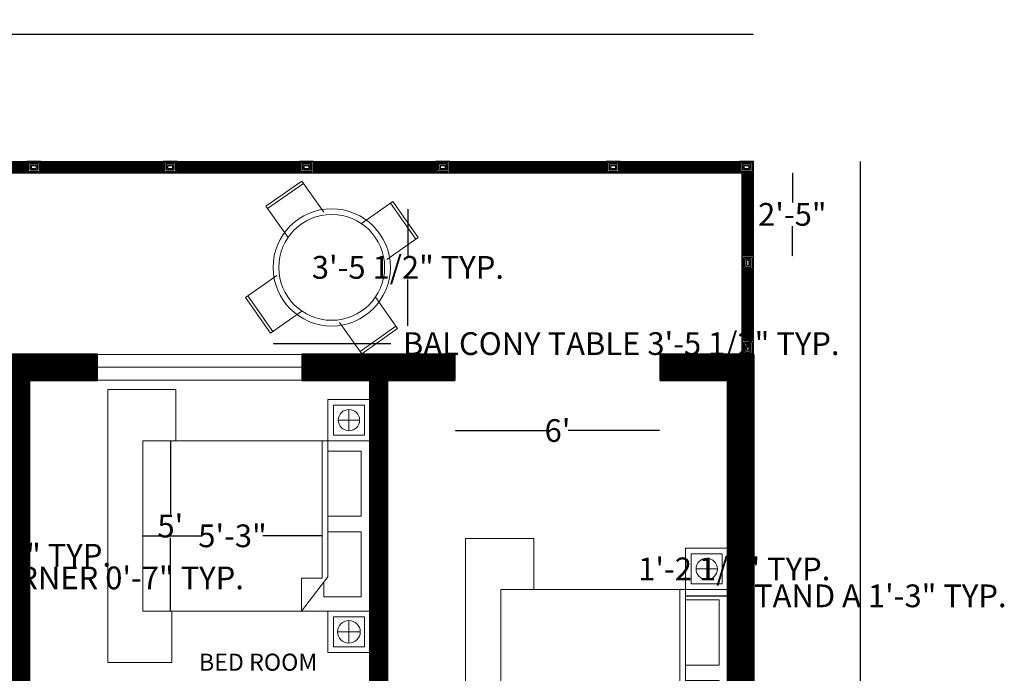
# Model space of a CAD drawing. Units: inches. Extents: x 348 to 1197, y 2602 to 3078.
# Tile 4 of 4: x 850 to 1197, y 2848 to 3078. Entities that reach past the tile are written whole.
import ezdxf

# ---------------------------------------------------------------- set-up
doc = ezdxf.new("R2010")
doc.units = ezdxf.units.IN
doc.header["$MEASUREMENT"] = 0
for name, color, linetype, lineweight in [('A-ANNO-DIMS', 20, 'Continuous', 18), ('A-AREA-IDEN', 104, 'Continuous', 18), ('A-WALL-PATT', 250, 'Continuous', 13), ('balcony', 201, 'Continuous', 25), ('bed', 5, 'Continuous', 18), ('table', 6, 'Continuous', 18), ('walls', 4, 'Continuous', 50), ('windows', 2, 'Continuous', 18)]:
    doc.layers.add(name, color=color, linetype=linetype, lineweight=lineweight)
doc.styles.get("Standard").update_dxf_attribs({"font": 'arial.ttf'})
doc.dimstyles.get("Standard").update_dxf_attribs({"dimtxt": 8, "dimasz": 0.18, "dimexe": 0.18, "dimexo": 0.0625, "dimgap": 0.09, "dimtad": 0, "dimtih": 1, "dimtoh": 1, "dimdec": 0, "dimzin": 0, "dimdsep": 46, "dimlunit": 3, "dimtxsty": 'Standard', "dimblk": 'DOT', "dimcen": 0.09, "dimse1": 1, "dimse2": 1, "dimadec": 0, "dimazin": 0, "dimtfac": 1, "dimtdec": 0, "dimtofl": 0, "dimtmove": 0, "dimatfit": 3, "dimfxl": 1, "dimtolj": 1, "dimtzin": 0, "dimarcsym": 0})

# ---------------------------------------------------------------- blocks, each defined once
blk = doc.blocks.new('*U16')
at = {"layer": 'table'}
for p, q in [((-7.7, -6.73), (-7.7, 6.73)), ((-7.7, 6.73), (7.7, 6.73)), ((-7.7, 5.73), (7.7, 5.73)), ((7.7, 6.73), (7.7, -6.73))]:
    blk.add_line(p, q, dxfattribs=at)
blk = doc.blocks.new('*U17')
at = {"layer": 'table', "transparency": 16777216}
blk.add_blockref('*U16', (596.31, 3015.18), dxfattribs=at)
for p, rotation in [((570.95, 2992.17), 90), ((619.32, 2989.82), 270), ((593.96, 2966.81), 180)]:
    blk.add_blockref('*U16', p, dxfattribs=dict(at, rotation=rotation))
blk = doc.blocks.new('_Dot')
at = {"color": 0, "linetype": 'ByBlock', "lineweight": -2}
blk.add_line((-0.5, 0), (-1, 0), dxfattribs=at)
at = {"color": 0, "linetype": 'ByBlock', "const_width": 0.5}
blk.add_lwpolyline([(-0.25, 0, 1), (0.25, 0, 1)], format="xyb", close=True, dxfattribs=at)
blk = doc.blocks.new('*D21')
at = {"layer": 'A-ANNO-DIMS', "color": 0, "lineweight": -2, "transparency": 16777216}
for p, q in [((1122, 3023.99), (1122, 3013.7)), ((1122, 2995.07), (1122, 3005.35))]:
    blk.add_line(p, q, dxfattribs=at)
at = {"layer": 'Defpoints', "color": 0, "transparency": 16777216}
for p in [(1108.32, 3024.17), (1122, 3024.17), (1108.32, 2994.89)]:
    blk.add_point(p, dxfattribs=at)
at = {"layer": 'A-ANNO-DIMS', "color": 0, "lineweight": -2, "transparency": 16777216, "xscale": 0.18, "yscale": 0.18, "zscale": 0.18}
for p, rotation in [((1122, 3024.17), 90), ((1122, 2994.89), 270)]:
    blk.add_blockref('_Dot', p, dxfattribs=dict(at, rotation=rotation))
at = {"layer": 'A-ANNO-DIMS', "color": 0, "transparency": 16777216, "insert": (1122, 3009.53), "char_height": 8, "attachment_point": 5}
blk.add_mtext('\\A1;2\'-5"', dxfattribs=at)
blk = doc.blocks.new('*D22')
at = {"layer": 'A-ANNO-DIMS', "color": 0, "lineweight": -2, "transparency": 16777216}
for p, q in [((1003.5, 2933.44), (1035.52, 2933.44)), ((1075.14, 2933.44), (1043.11, 2933.44))]:
    blk.add_line(p, q, dxfattribs=at)
at = {"layer": 'Defpoints', "color": 0, "transparency": 16777216}
for p in [(1003.32, 2955.7), (1075.32, 2955.7), (1003.32, 2933.44)]:
    blk.add_point(p, dxfattribs=at)
at = {"layer": 'A-ANNO-DIMS', "color": 0, "lineweight": -2, "transparency": 16777216, "xscale": 0.18, "yscale": 0.18, "zscale": 0.18, "rotation": 180}
blk.add_blockref('_Dot', (1003.32, 2933.44), dxfattribs=at)
at = {"layer": 'A-ANNO-DIMS', "color": 0, "lineweight": -2, "transparency": 16777216, "xscale": 0.18, "yscale": 0.18, "zscale": 0.18}
blk.add_blockref('_Dot', (1075.32, 2933.44), dxfattribs=at)
at = {"layer": 'A-ANNO-DIMS', "color": 0, "transparency": 16777216, "insert": (1039.32, 2933.44), "char_height": 8, "attachment_point": 5}
blk.add_mtext("\\A1;6'", dxfattribs=at)
blk = doc.blocks.new('*D33')
at = {"layer": 'A-ANNO-DIMS', "color": 0, "lineweight": -2, "transparency": 16777216}
for p, q in [((893.5, 2896.39), (914.14, 2896.39)), ((956.24, 2896.39), (935.59, 2896.39))]:
    blk.add_line(p, q, dxfattribs=at)
at = {"layer": 'Defpoints', "color": 0, "transparency": 16777216}
for p in [(893.32, 2899.84), (956.42, 2896.39), (956.42, 2896.39)]:
    blk.add_point(p, dxfattribs=at)
at = {"layer": 'A-ANNO-DIMS', "color": 0, "lineweight": -2, "transparency": 16777216, "xscale": 0.18, "yscale": 0.18, "zscale": 0.18, "rotation": 180}
blk.add_blockref('_Dot', (893.32, 2896.39), dxfattribs=at)
at = {"layer": 'A-ANNO-DIMS', "color": 0, "lineweight": -2, "transparency": 16777216, "xscale": 0.18, "yscale": 0.18, "zscale": 0.18}
blk.add_blockref('_Dot', (956.42, 2896.39), dxfattribs=at)
at = {"layer": 'A-ANNO-DIMS', "color": 0, "transparency": 16777216, "insert": (924.87, 2896.39), "char_height": 8, "attachment_point": 5}
blk.add_mtext('\\A1;5\'-3"', dxfattribs=at)
blk = doc.blocks.new('*D34')
at = {"layer": 'A-ANNO-DIMS', "color": 0, "lineweight": -2, "transparency": 16777216}
for p, q in [((902.98, 2929.66), (902.98, 2903.99)), ((902.98, 2870.02), (902.98, 2895.68))]:
    blk.add_line(p, q, dxfattribs=at)
at = {"layer": 'Defpoints', "color": 0, "transparency": 16777216}
for p in [(902.98, 2929.84), (933.32, 2929.84), (937.33, 2869.84)]:
    blk.add_point(p, dxfattribs=at)
at = {"layer": 'A-ANNO-DIMS', "color": 0, "lineweight": -2, "transparency": 16777216, "xscale": 0.18, "yscale": 0.18, "zscale": 0.18}
for p, rotation in [((902.98, 2929.84), 90), ((902.98, 2869.84), 270)]:
    blk.add_blockref('_Dot', p, dxfattribs=dict(at, rotation=rotation))
at = {"layer": 'A-ANNO-DIMS', "color": 0, "transparency": 16777216, "insert": (902.98, 2899.84), "char_height": 8, "attachment_point": 5}
blk.add_mtext("\\A1;5'", dxfattribs=at)
blk = doc.blocks.new('BED-QUEEN')
for p, q in [((24, 96), (0, 96)), ((0, 96), (0, 0)), ((24, 78), (24, 96)), ((92.39, 78), (12.39, 78)), ((12.39, 78), (12.39, 18)), ((75.49, 78), (75.49, 29.69)), ((77.49, 78), (77.49, 30.16)), ((77.49, 30.16), (68.23, 18)), ((68.23, 29.62), (75.49, 29.69)), ((68.23, 18), (68.23, 29.62)), ((12.39, 18), (92.39, 18)), ((22.56, 18), (22.56, 0)), ((22.56, 0), (0, 0))]:
    blk.add_line(p, q)
for points in [[(77.49, 51.42), (89.26, 51.42), (89.26, 74.34), (77.49, 74.34)], [(76.09, 28.32), (76.09, 23.06), (89.26, 23.06), (89.26, 45.98), (77.49, 45.98)]]:
    blk.add_lwpolyline(points)
blk = doc.blocks.new('NIGHTSTAND-LAMP-A')
for p, q in [((7.45, 11), (7.45, 3.51)), ((3.7, 7.26), (11.2, 7.26))]:
    blk.add_line(p, q)
for points in [[(14.9, 0), (0, 0), (0, 14.51), (14.9, 14.51)], [(12.9, 2), (2, 2), (2, 12.51), (12.9, 12.51)]]:
    blk.add_lwpolyline(points, close=True)
blk.add_circle((7.45, 7.26), 3.75)
blk = doc.blocks.new('NIGHTSTAND-LAMP-B')
for p, q in [((7.45, 11.24), (7.45, 3.27)), ((11.44, 7.26), (3.46, 7.26))]:
    blk.add_line(p, q)
for points in [[(14.9, 0), (0, 0), (0, 14.51), (14.9, 14.51)], [(12.9, 2), (2, 2), (2, 12.51), (12.9, 12.51)]]:
    blk.add_lwpolyline(points, close=True)
blk.add_circle((7.45, 7.26), 3.99)
blk = doc.blocks.new('RAIL-POST-CORE')
for points in [[(0, 0), (3, 0), (3, 3.9), (0, 3.9)], [(0.5, 0.5), (2.5, 0.5), (2.5, 3.4), (0.5, 3.4)], [(1, 1), (2, 1), (2, 2.9), (1, 2.9)]]:
    blk.add_lwpolyline(points, close=True)
blk = doc.blocks.new('BALCONY-TABLE-ROUND')
for radius in [20.64, 18.64]:
    blk.add_circle((20.64, 20.64), radius)
blk = doc.blocks.new('*D52')
at = {"layer": 'A-ANNO-DIMS', "color": 0, "lineweight": -2, "transparency": 16777216}
for p, q in [((939.34, 2964.05), (980.26, 2964.05)), ((980.44, 2964.05), (980.62, 2964.05))]:
    blk.add_line(p, q, dxfattribs=at)
at = {"layer": 'Defpoints', "color": 0, "transparency": 16777216}
for p in [(939.16, 2970.24), (980.44, 2970.24), (980.44, 2964.05)]:
    blk.add_point(p, dxfattribs=at)
at = {"layer": 'A-ANNO-DIMS', "color": 0, "lineweight": -2, "transparency": 16777216, "xscale": 0.18, "yscale": 0.18, "zscale": 0.18, "rotation": 180}
blk.add_blockref('_Dot', (939.16, 2964.05), dxfattribs=at)
at = {"layer": 'A-ANNO-DIMS', "color": 0, "lineweight": -2, "transparency": 16777216, "xscale": 0.18, "yscale": 0.18, "zscale": 0.18}
blk.add_blockref('_Dot', (980.44, 2964.05), dxfattribs=at)
at = {"layer": 'A-ANNO-DIMS', "color": 0, "transparency": 16777216, "insert": (1061.75, 2964.05), "char_height": 8, "attachment_point": 5}
blk.add_mtext('\\A1;BALCONY TABLE 3\'-5 1/2" TYP.', dxfattribs=at)
blk = doc.blocks.new('*D53')
at = {"layer": 'A-ANNO-DIMS', "color": 0, "lineweight": -2, "transparency": 16777216}
for p, q in [((986.63, 3011.33), (986.63, 2995.1)), ((986.63, 2970.42), (986.63, 2986.65))]:
    blk.add_line(p, q, dxfattribs=at)
at = {"layer": 'Defpoints', "color": 0, "transparency": 16777216}
for p in [(980.44, 3011.51), (986.63, 3011.51), (980.44, 2970.24)]:
    blk.add_point(p, dxfattribs=at)
at = {"layer": 'A-ANNO-DIMS', "color": 0, "lineweight": -2, "transparency": 16777216, "xscale": 0.18, "yscale": 0.18, "zscale": 0.18}
for p, rotation in [((986.63, 3011.51), 90), ((986.63, 2970.24), 270)]:
    blk.add_blockref('_Dot', p, dxfattribs=dict(at, rotation=rotation))
at = {"layer": 'A-ANNO-DIMS', "color": 0, "transparency": 16777216, "insert": (986.63, 2990.88), "char_height": 8, "attachment_point": 5}
blk.add_mtext('\\A1;3\'-5 1/2" TYP.', dxfattribs=at)
blk = doc.blocks.new('*D62')
at = {"layer": 'A-ANNO-DIMS', "color": 0, "lineweight": -2, "transparency": 16777216}
for p, q in [((825.4, 2881.58), (831.83, 2881.58)), ((832.01, 2881.58), (832.19, 2881.58))]:
    blk.add_line(p, q, dxfattribs=at)
at = {"layer": 'Defpoints', "color": 0, "transparency": 16777216}
for p in [(825.22, 2882.6), (832.01, 2882.6), (832.01, 2881.58)]:
    blk.add_point(p, dxfattribs=at)
at = {"layer": 'A-ANNO-DIMS', "color": 0, "lineweight": -2, "transparency": 16777216, "xscale": 0.18, "yscale": 0.18, "zscale": 0.18, "rotation": 180}
blk.add_blockref('_Dot', (825.22, 2881.58), dxfattribs=at)
at = {"layer": 'A-ANNO-DIMS', "color": 0, "lineweight": -2, "transparency": 16777216, "xscale": 0.18, "yscale": 0.18, "zscale": 0.18}
blk.add_blockref('_Dot', (832.01, 2881.58), dxfattribs=at)
at = {"layer": 'A-ANNO-DIMS', "color": 0, "transparency": 16777216, "insert": (881.63, 2881.58), "char_height": 8, "attachment_point": 5}
blk.add_mtext('\\A1;BURNER 0\'-7" TYP.', dxfattribs=at)
blk = doc.blocks.new('*D63')
at = {"layer": 'A-ANNO-DIMS', "color": 0, "lineweight": -2, "transparency": 16777216}
for p, q in [((833.03, 2889.38), (833.03, 2889.56)), ((833.03, 2889.56), (833.21, 2889.56)), ((833.03, 2882.78), (833.03, 2889.2))]:
    blk.add_line(p, q, dxfattribs=at)
at = {"layer": 'Defpoints', "color": 0, "transparency": 16777216}
for p in [(832.01, 2889.38), (833.03, 2889.38), (832.01, 2882.6)]:
    blk.add_point(p, dxfattribs=at)
at = {"layer": 'A-ANNO-DIMS', "color": 0, "lineweight": -2, "transparency": 16777216, "xscale": 0.18, "yscale": 0.18, "zscale": 0.18}
for p, rotation in [((833.03, 2889.38), 90), ((833.03, 2882.6), 270)]:
    blk.add_blockref('_Dot', p, dxfattribs=dict(at, rotation=rotation))
at = {"layer": 'A-ANNO-DIMS', "color": 0, "transparency": 16777216, "insert": (857.68, 2889.56), "char_height": 8, "attachment_point": 5}
blk.add_mtext('\\A1;0\'-7" TYP.', dxfattribs=at)
blk = doc.blocks.new('*D64')
at = {"layer": 'A-ANNO-DIMS', "color": 0, "lineweight": -2, "transparency": 16777216}
for p, q in [((1084.6, 2875.26), (1099.14, 2875.26)), ((1099.32, 2875.26), (1099.5, 2875.26))]:
    blk.add_line(p, q, dxfattribs=at)
at = {"layer": 'Defpoints', "color": 0, "transparency": 16777216}
for p in [(1084.42, 2877.5), (1099.32, 2877.5), (1099.32, 2875.26)]:
    blk.add_point(p, dxfattribs=at)
at = {"layer": 'A-ANNO-DIMS', "color": 0, "lineweight": -2, "transparency": 16777216, "xscale": 0.18, "yscale": 0.18, "zscale": 0.18, "rotation": 180}
blk.add_blockref('_Dot', (1084.42, 2875.26), dxfattribs=at)
at = {"layer": 'A-ANNO-DIMS', "color": 0, "lineweight": -2, "transparency": 16777216, "xscale": 0.18, "yscale": 0.18, "zscale": 0.18}
blk.add_blockref('_Dot', (1099.32, 2875.26), dxfattribs=at)
at = {"layer": 'A-ANNO-DIMS', "color": 0, "transparency": 16777216, "insert": (1149.72, 2875.26), "char_height": 8, "attachment_point": 5}
blk.add_mtext('\\A1;STAND A 1\'-3" TYP.', dxfattribs=at)
blk = doc.blocks.new('*D65')
at = {"layer": 'A-ANNO-DIMS', "color": 0, "lineweight": -2, "transparency": 16777216}
for p, q in [((1101.55, 2891.83), (1101.55, 2888.98)), ((1101.55, 2877.68), (1101.55, 2880.52))]:
    blk.add_line(p, q, dxfattribs=at)
at = {"layer": 'Defpoints', "color": 0, "transparency": 16777216}
for p in [(1099.32, 2892.01), (1101.55, 2892.01), (1099.32, 2877.5)]:
    blk.add_point(p, dxfattribs=at)
at = {"layer": 'A-ANNO-DIMS', "color": 0, "lineweight": -2, "transparency": 16777216, "xscale": 0.18, "yscale": 0.18, "zscale": 0.18}
for p, rotation in [((1101.55, 2892.01), 90), ((1101.55, 2877.5), 270)]:
    blk.add_blockref('_Dot', p, dxfattribs=dict(at, rotation=rotation))
at = {"layer": 'A-ANNO-DIMS', "color": 0, "transparency": 16777216, "insert": (1101.55, 2884.75), "char_height": 8, "attachment_point": 5}
blk.add_mtext('\\A1;1\'-2 1/2" TYP.', dxfattribs=at)
blk = doc.blocks.new('*D68')
at = {"layer": 'A-ANNO-DIMS', "color": 0, "lineweight": -2, "transparency": 16777216}
for p, q in [((399.5, 3072.8), (739.99, 3072.8)), ((1108.14, 3072.8), (767.65, 3072.8))]:
    blk.add_line(p, q, dxfattribs=at)
at = {"layer": 'Defpoints', "color": 0, "transparency": 16777216}
for p in [(1108.32, 3072.8), (1108.32, 3028.2), (399.32, 3018.2)]:
    blk.add_point(p, dxfattribs=at)
at = {"layer": 'A-ANNO-DIMS', "color": 0, "lineweight": -2, "transparency": 16777216, "xscale": 0.18, "yscale": 0.18, "zscale": 0.18, "rotation": 180}
blk.add_blockref('_Dot', (399.32, 3072.8), dxfattribs=at)
at = {"layer": 'A-ANNO-DIMS', "color": 0, "lineweight": -2, "transparency": 16777216, "xscale": 0.18, "yscale": 0.18, "zscale": 0.18}
blk.add_blockref('_Dot', (1108.32, 3072.8), dxfattribs=at)
at = {"layer": 'A-ANNO-DIMS', "color": 0, "transparency": 16777216, "insert": (753.82, 3072.8), "char_height": 8, "attachment_point": 5}
blk.add_mtext('\\A1;59\'-1"', dxfattribs=at)
blk = doc.blocks.new('*D69')
at = {"layer": 'A-ANNO-DIMS', "color": 0, "lineweight": -2, "transparency": 16777216}
for p, q in [((1145.87, 3028.02), (1145.87, 2840.88)), ((1145.87, 2645.38), (1145.87, 2832.53))]:
    blk.add_line(p, q, dxfattribs=at)
at = {"layer": 'Defpoints', "color": 0, "transparency": 16777216}
for p in [(1108.32, 3028.2), (1145.87, 3028.2), (1108.32, 2645.2)]:
    blk.add_point(p, dxfattribs=at)
at = {"layer": 'A-ANNO-DIMS', "color": 0, "lineweight": -2, "transparency": 16777216, "xscale": 0.18, "yscale": 0.18, "zscale": 0.18}
for p, rotation in [((1145.87, 3028.2), 90), ((1145.87, 2645.2), 270)]:
    blk.add_blockref('_Dot', p, dxfattribs=dict(at, rotation=rotation))
at = {"layer": 'A-ANNO-DIMS', "color": 0, "transparency": 16777216, "insert": (1145.87, 2836.7), "char_height": 8, "attachment_point": 5}
blk.add_mtext('\\A1;31\'-11"', dxfattribs=at)
blk = doc.blocks.new('*D81')
at = {"layer": 'A-ANNO-DIMS', "color": 0, "lineweight": -2, "transparency": 16777216}
for p, q in [((877.5, 2607.65), (902.57, 2607.65)), ((949.14, 2607.65), (924.06, 2607.65))]:
    blk.add_line(p, q, dxfattribs=at)
at = {"layer": 'Defpoints', "color": 0, "transparency": 16777216}
for p in [(877.32, 2951.2), (949.32, 2951.2), (949.32, 2607.65)]:
    blk.add_point(p, dxfattribs=at)
at = {"layer": 'A-ANNO-DIMS', "color": 0, "lineweight": -2, "transparency": 16777216, "xscale": 0.18, "yscale": 0.18, "zscale": 0.18, "rotation": 180}
blk.add_blockref('_Dot', (877.32, 2607.65), dxfattribs=at)
at = {"layer": 'A-ANNO-DIMS', "color": 0, "lineweight": -2, "transparency": 16777216, "xscale": 0.18, "yscale": 0.18, "zscale": 0.18}
blk.add_blockref('_Dot', (949.32, 2607.65), dxfattribs=at)
at = {"layer": 'A-ANNO-DIMS', "color": 0, "transparency": 16777216, "insert": (913.32, 2607.65), "char_height": 8, "attachment_point": 5}
blk.add_mtext('\\A1;6\'-0"', dxfattribs=at)

msp = doc.modelspace()

# ---------------------------------------------------------------- hatches: boundary and pattern name
at = {"layer": 'A-WALL-PATT'}
h = msp.add_hatch(dxfattribs=at)
h.set_pattern_fill('ANSI31', color=256, scale=1.5)
h.paths.add_polyline_path([(481.32, 2951.2), (509.32, 2951.2), (509.32, 2960.2), (505.32, 2960.2), (481.32, 2960.2), (481.32, 3018.2), (452.32, 3018.2), (452.32, 3009.2), (472.32, 3009.2), (472.32, 2943.2), (481.32, 2943.2)], flags=17)
h.paths.add_polyline_path([(428.32, 3018.2), (399.32, 3018.2), (399.32, 2904.2), (472.32, 2904.2), (472.32, 2726.2), (532.32, 2726.2), (532.32, 2696.2), (541.32, 2696.2), (541.32, 2726.2), (565.32, 2726.2), (565.32, 2735.2), (481.32, 2735.2), (481.32, 2758.72), (481.32, 2809.83), (481.31, 2809.83), (481.31, 2824.34), (481.31, 2884.34), (481.31, 2884.34), (481.31, 2898.86), (481.32, 2913.2), (472.32, 2913.2), (408.32, 2913.2), (408.32, 3009.2), (428.32, 3009.2)])
h.paths.add_polyline_path([(796.32, 2654.2), (769.32, 2654.2), (769.32, 2753.2), (769.32, 2759.2), (763.32, 2759.2), (763.32, 2735.2), (763.32, 2654.2), (541.32, 2654.2), (532.32, 2654.2), (532.32, 2645.2), (796.32, 2645.2)])
h.paths.add_polyline_path([(853.32, 2726.2), (1018.32, 2726.2), (1018.32, 2703.7), (1027.32, 2703.7), (1027.32, 2729.2), (1057.32, 2729.2), (1057.32, 2735.2), (919.32, 2735.2), (919.32, 2758.72), (919.32, 2765.2), (913.32, 2765.2), (913.32, 2735.2), (853.32, 2735.2), (853.32, 2759.2), (799.32, 2759.2), (799.32, 2753.2), (847.32, 2753.2), (847.32, 2654.2), (820.32, 2654.2), (820.32, 2645.2), (853.32, 2645.2)])
h.paths.add_polyline_path([(640.32, 2960.2), (577.32, 2960.2), (577.32, 2951.2), (601.32, 2951.2), (601.32, 2735.2), (601.32, 2726.2), (607.32, 2726.2), (607.32, 2951.2), (640.32, 2951.2)])
h.paths.add_polyline_path([(877.32, 2960.2), (688.32, 2960.2), (688.32, 2951.2), (745.32, 2951.2), (745.32, 2837.2), (751.32, 2837.2), (751.32, 2951.2), (847.32, 2951.2), (847.32, 2807.2), (751.32, 2807.2), (745.32, 2807.2), (745.32, 2801.2), (853.32, 2801.2), (853.32, 2807.2), (853.32, 2951.2), (877.32, 2951.2)])
h.paths.add_polyline_path([(1003.32, 2960.2), (949.32, 2960.2), (949.32, 2951.2), (973.32, 2951.2), (973.32, 2807.2), (906.15, 2807.2), (893.32, 2807.2), (893.32, 2801.2), (913.32, 2801.2), (919.32, 2801.2), (955.32, 2801.2), (979.32, 2801.2), (979.32, 2951.2), (1003.32, 2951.2)])
h.paths.add_polyline_path([(1108.32, 2960.2), (1104.32, 2960.2), (1075.32, 2960.2), (1075.32, 2951.2), (1099.32, 2951.2), (1099.32, 2735.2), (1087.32, 2735.2), (1087.32, 2729.2), (1099.32, 2729.2), (1099.32, 2654.2), (1027.32, 2654.2), (1027.32, 2679.7), (1018.32, 2679.7), (1018.32, 2645.2), (1108.32, 2645.2)])
h.paths.add_polyline_path([(509.32, 2992.2), (505.32, 2992.2), (505.32, 2965.1), (509.32, 2965.1)], flags=16)
h.paths.add_polyline_path([(509.32, 3023.27), (505.32, 3023.27), (505.32, 2997.1), (509.32, 2997.1)])
h.paths.add_polyline_path([(576.46, 3028.2), (509.32, 3028.2), (509.32, 3024.2), (576.46, 3024.2)])
h.paths.add_polyline_path([(624.46, 3028.2), (581.36, 3028.2), (581.36, 3024.2), (624.46, 3024.2)])
h.paths.add_polyline_path([(672.46, 3028.2), (629.36, 3028.2), (629.36, 3024.2), (672.46, 3024.2)])
h.paths.add_polyline_path([(720.46, 3028.2), (677.36, 3028.2), (677.36, 3024.2), (720.46, 3024.2)])
h.paths.add_polyline_path([(768.46, 3028.2), (725.36, 3028.2), (725.36, 3024.2), (768.46, 3024.2)])
h.paths.add_polyline_path([(804.46, 3028.2), (773.36, 3028.2), (773.36, 3024.2), (804.46, 3024.2)])
h.paths.add_polyline_path([(852.46, 3028.2), (809.36, 3028.2), (809.36, 3024.2), (852.46, 3024.2)])
h.paths.add_polyline_path([(900.46, 3028.2), (857.36, 3028.2), (857.36, 3024.2), (900.46, 3024.2)])
h.paths.add_polyline_path([(948.46, 3028.2), (905.36, 3028.2), (905.36, 3024.2), (948.46, 3024.2)])
h.paths.add_polyline_path([(996.46, 3028.2), (953.36, 3028.2), (953.36, 3024.2), (996.46, 3024.2)])
h.paths.add_polyline_path([(1056.46, 3028.2), (1001.36, 3028.2), (1001.36, 3024.2), (1056.46, 3024.2)])
h.paths.add_polyline_path([(1103.42, 3028.2), (1061.36, 3028.2), (1061.36, 3024.2), (1103.42, 3024.2)])
h.paths.add_polyline_path([(1108.32, 3024.17), (1104.32, 3024.17), (1104.32, 2994.89), (1108.32, 2994.89)])
h.paths.add_polyline_path([(1108.32, 2989.99), (1104.32, 2989.99), (1104.32, 2965.1), (1108.32, 2965.1)])

# ---------------------------------------------------------------- linework, layer by layer
at = {"layer": 'balcony'}
for p, q in [((505.32, 3028.2), (1108.32, 3028.2)), ((1108.32, 2960.2), (1108.32, 3028.2)), ((509.32, 3024.2), (1104.32, 3024.2)), ((1104.32, 2960.2), (1104.32, 3024.2))]:
    msp.add_line(p, q, dxfattribs=at)
for points in [[(857.36, 3024.17), (857.36, 3028.17), (852.46, 3028.17), (852.46, 3024.17)], [(905.36, 3024.17), (905.36, 3028.17), (900.46, 3028.17), (900.46, 3024.17)], [(953.36, 3024.17), (953.36, 3028.17), (948.46, 3028.17), (948.46, 3024.17)], [(1001.36, 3024.17), (1001.36, 3028.17), (996.46, 3028.17), (996.46, 3024.17)], [(1061.36, 3024.17), (1061.36, 3028.17), (1056.46, 3028.17), (1056.46, 3024.17)], [(1108.32, 3024.17), (1108.32, 3028.17), (1103.42, 3028.17), (1103.42, 3024.17)], [(1104.32, 2989.99), (1108.32, 2989.99), (1108.32, 2994.89), (1104.32, 2994.89)], [(1104.32, 2960.2), (1108.32, 2960.2), (1108.32, 2965.1), (1104.32, 2965.1)]]:
    msp.add_lwpolyline(points, close=True, dxfattribs=at)
at = {"layer": 'bed'}
for p, q in [((904.92, 2947.84), (880.92, 2947.84)), ((880.92, 2947.84), (880.92, 2851.84)), ((904.92, 2929.84), (904.92, 2947.84)), ((973.32, 2929.84), (893.32, 2929.84)), ((893.32, 2929.84), (893.32, 2869.84)), ((956.42, 2929.84), (956.42, 2881.53)), ((958.42, 2929.84), (958.42, 2882)), ((958.42, 2882), (949.15, 2869.84)), ((949.15, 2881.46), (956.42, 2881.53)), ((949.15, 2869.84), (949.15, 2881.46)), ((893.32, 2869.84), (973.32, 2869.84)), ((903.48, 2869.84), (903.48, 2851.84)), ((903.48, 2851.84), (880.92, 2851.84))]:
    msp.add_line(p, q, dxfattribs=at)
for points in [[(958.42, 2903.26), (970.19, 2903.26), (970.19, 2926.18), (958.42, 2926.18)], [(957.01, 2880.15), (957.01, 2874.9), (970.19, 2874.9), (970.19, 2897.81), (958.42, 2897.81)]]:
    msp.add_lwpolyline(points, dxfattribs=at)
at = {"layer": 'walls'}
for p, q in [((688.32, 2960.2), (877.32, 2960.2)), ((949.32, 2960.2), (1003.32, 2960.2)), ((1075.32, 2960.2), (1104.32, 2960.2)), ((1108.32, 2960.2), (1108.32, 2645.2)), ((853.32, 2951.2), (853.32, 2807.2)), ((853.32, 2951.2), (877.32, 2951.2)), ((949.32, 2951.2), (973.32, 2951.2)), ((973.32, 2951.2), (973.32, 2807.2)), ((979.32, 2951.2), (979.32, 2801.2)), ((979.32, 2951.2), (1003.32, 2951.2)), ((1075.32, 2951.2), (1099.32, 2951.2)), ((1099.32, 2951.2), (1099.32, 2735.2))]:
    msp.add_line(p, q, dxfattribs=at)
at = {"layer": 'windows'}
for p, q in [((877.32, 2951.2), (877.32, 2960.2)), ((877.32, 2960.2), (949.32, 2960.2)), ((949.32, 2951.2), (949.32, 2960.2)), ((1003.32, 2951.2), (1003.32, 2960.2)), ((1075.32, 2951.2), (1075.32, 2960.2)), ((877.32, 2955.7), (949.32, 2955.7)), ((877.32, 2951.2), (949.32, 2951.2))]:
    msp.add_line(p, q, dxfattribs=at)

# ---------------------------------------------------------------- block references
at = {"layer": 'balcony'}
for p, rotation in [((856.86, 3024.67), 90.0000000000149), ((904.86, 3024.67), 90.00000000001351), ((952.86, 3024.67), 90.00000000001351), ((1000.86, 3024.67), 90.00000000001351), ((1060.86, 3024.67), 90.0000000000149), ((1107.82, 3024.67), 90.0000000000177)]:
    msp.add_blockref('RAIL-POST-CORE', p, dxfattribs=dict(at, rotation=rotation))
for p in [(1104.82, 2990.49), (1104.82, 2960.7)]:
    msp.add_blockref('RAIL-POST-CORE', p, dxfattribs=at)
at = {"layer": 'bed'}
for name, p in [('NIGHTSTAND-LAMP-A', (958.41, 2929.84)), ('BED-QUEEN', (1006.92, 2799.49)), ('NIGHTSTAND-LAMP-A', (1084.41, 2877.49)), ('NIGHTSTAND-LAMP-B', (958.41, 2855.32))]:
    msp.add_blockref(name, p, dxfattribs=at)
at = {"layer": 'table', "rotation": 215.168770522954}
msp.add_blockref('*U17', (-276.47, 5778.68), dxfattribs=at)
at = {"layer": 'table'}
msp.add_blockref('BALCONY-TABLE-ROUND', (939.17, 2970.24), dxfattribs=at)

# ---------------------------------------------------------------- texts
at = {"layer": 'A-AREA-IDEN'}
msp.add_text('BED ROOM ', height=6, dxfattribs=at).set_placement((913.05, 2848.91))

# ---------------------------------------------------------------- dimensions: what is measured, and where the dimension line sits
at = {"layer": 'A-ANNO-DIMS'}
for base, p1, p2, override, picture, middle in [((1108.32, 3072.8), (399.32, 3018.2), (1108.32, 3028.2), {"dimdec": 1, "dimlfac": 1, "dimrnd": 0, "dimzin": 1, "dimdsep": 46, "dimlunit": 4, "dimfrac": 2}, '*D68', (753.82, 3072.8)), ((1003.32, 2933.44), (1075.32, 2955.7), (1003.32, 2955.7), {"dimclrd": 0, "dimclre": 0, "dimclrt": 0}, '*D22', (1039.32, 2933.44)), ((949.32, 2607.65), (877.32, 2951.2), (949.32, 2951.2), {"dimdec": 1, "dimlfac": 1, "dimrnd": 0, "dimzin": 1, "dimdsep": 46, "dimlunit": 4, "dimfrac": 2}, '*D81', (913.32, 2607.65)), ((956.42, 2896.39), (893.32, 2899.84), (956.42, 2896.39), {"dimclrd": 0, "dimclre": 0, "dimclrt": 0}, '*D33', (924.87, 2896.39))]:
    dim = msp.add_linear_dim(base=base, p1=p1, p2=p2, dimstyle='Standard', override=override, dxfattribs=at)
    dim.commit()
    dim.dimension.update_dxf_attribs({"geometry": picture, "text_midpoint": middle})
for base, p1, p2, override, picture, middle in [((1145.87, 3028.2), (1108.32, 2645.2), (1108.32, 3028.2), {"dimdec": 1, "dimlfac": 1, "dimrnd": 0, "dimzin": 1, "dimdsep": 46, "dimlunit": 4, "dimfrac": 2}, '*D69', (1145.87, 2836.7)), ((1122, 3024.17), (1108.32, 2994.89), (1108.32, 3024.17), {"dimclrd": 0, "dimclre": 0, "dimclrt": 0}, '*D21', (1122, 3009.53)), ((902.98, 2929.84), (937.33, 2869.84), (933.32, 2929.84), {"dimclrd": 0, "dimclre": 0, "dimclrt": 0}, '*D34', (902.98, 2899.84))]:
    dim = msp.add_linear_dim(base=base, p1=p1, p2=p2, angle=90, dimstyle='Standard', override=override, dxfattribs=at)
    dim.commit()
    dim.dimension.update_dxf_attribs({"geometry": picture, "text_midpoint": middle})
for base, p1, p2, picture, middle in [((986.63, 3011.51), (980.44, 2970.24), (980.44, 3011.51), '*D53', (986.63, 2990.88)), ((1101.55, 2892.01), (1099.32, 2877.5), (1099.32, 2892.01), '*D65', (1101.55, 2884.75)), ((833.03, 2889.38), (832.01, 2882.6), (832.01, 2889.38), '*D63', (857.68, 2889.56))]:
    dim = msp.add_linear_dim(base=base, p1=p1, p2=p2, angle=90, text='<> TYP.', dimstyle='Standard', override={"dimdec": 1, "dimlfac": 1, "dimrnd": 0, "dimzin": 1, "dimdsep": 46, "dimlunit": 4, "dimfrac": 2}, dxfattribs=at)
    dim.commit()
    dim.dimension.update_dxf_attribs({"geometry": picture, "text_midpoint": middle})
for base, p1, p2, text, picture, middle in [((980.44, 2964.05), (939.16, 2970.24), (980.44, 2970.24), 'BALCONY TABLE <> TYP.', '*D52', (1061.75, 2964.05)), ((832.01, 2881.58), (825.22, 2882.6), (832.01, 2882.6), 'BURNER <> TYP.', '*D62', (881.63, 2881.58)), ((1099.32, 2875.26), (1084.42, 2877.5), (1099.32, 2877.5), 'STAND A <> TYP.', '*D64', (1149.72, 2875.26))]:
    dim = msp.add_linear_dim(base=base, p1=p1, p2=p2, text=text, dimstyle='Standard', override={"dimdec": 1, "dimlfac": 1, "dimrnd": 0, "dimzin": 1, "dimdsep": 46, "dimlunit": 4, "dimfrac": 2}, dxfattribs=at)
    dim.commit()
    dim.dimension.update_dxf_attribs({"geometry": picture, "text_midpoint": middle})

doc.saveas('drawing.dxf')
